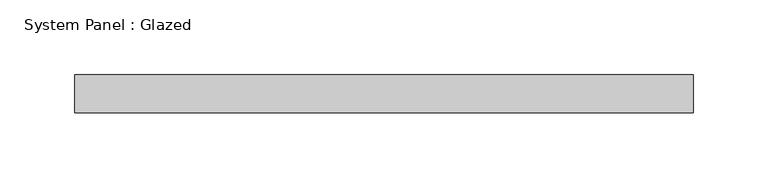
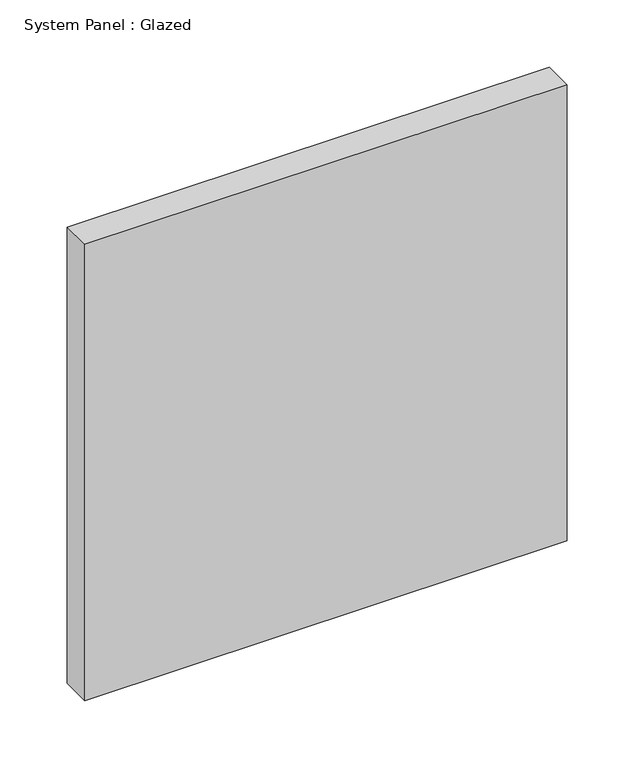
"""IFC4 building model written with IfcOpenShell, lengths in millimetres: plate geometry, System Panel : Glazed."""

from ifc_helpers import new_model, si_unit, origin, origin_with_axes, place, context, project, spatial, polyline, outline, extrude, source, transform, mapped, element, save


def system_panel_glazed_43ba880c(model_context):
    return source(origin(), model_context, "Body", "SweptSolid", [
        extrude(outline(polyline([(206.375, 19.05), (-206.375, 19.05), (-206.375, 44.45), (206.375, 44.45), (206.375, 19.05)])), origin_with_axes(), (0.0, 0.0, 1.0), 412.75),
    ])


if __name__ == "__main__":
    model = new_model("IFC4")
    model_context = context("Model", 3, world=origin())
    ifc_project = project(units=[si_unit("LENGTHUNIT", "METRE", prefix="MILLI")], contexts=[model_context])
    site = spatial("IfcSite", under=ifc_project)
    building = spatial("IfcBuilding", under=site)
    placement = place(None, origin())
    system_panel_glazed_shape = system_panel_glazed_43ba880c(model_context)
    element("IfcPlate", 1, ObjectType="System Panel : Glazed", at=placement, inside=building, context=model_context, shape_type="MappedRepresentation", body=[
        mapped(system_panel_glazed_shape, transform((0.0, 0.0, 0.0), x_axis=(1.0, 0.0, 0.0), y_axis=(0.0, 1.0, 0.0), z_axis=(0.0, 0.0, 1.0))),
    ])
    save(model, "model.ifc")

# Revit data of these elements
# Type "System Panel : Glazed"
#   Construction Type Id = "GSP4R"
#   Analytic Construction = "1/8 in Pilkington single glazing"
#   Visual Light Transmittance = 0.9
#   Solar Heat Gain Coefficient = 0.86
#   Heat Transfer Coefficient (U) = 1.18115 BTU/(h·ft²·°F)
#   Define Thermal Properties by = 1
# Element 1 (IfcPlate, "System Panel : Glazed")
#   Materials on its faces: "Glass"
# Materials
#   "Glass": class "Glass", colour RGB 0 128 192, transparency 0.75, Description = "Soda Lime Glass", Cost = 0
